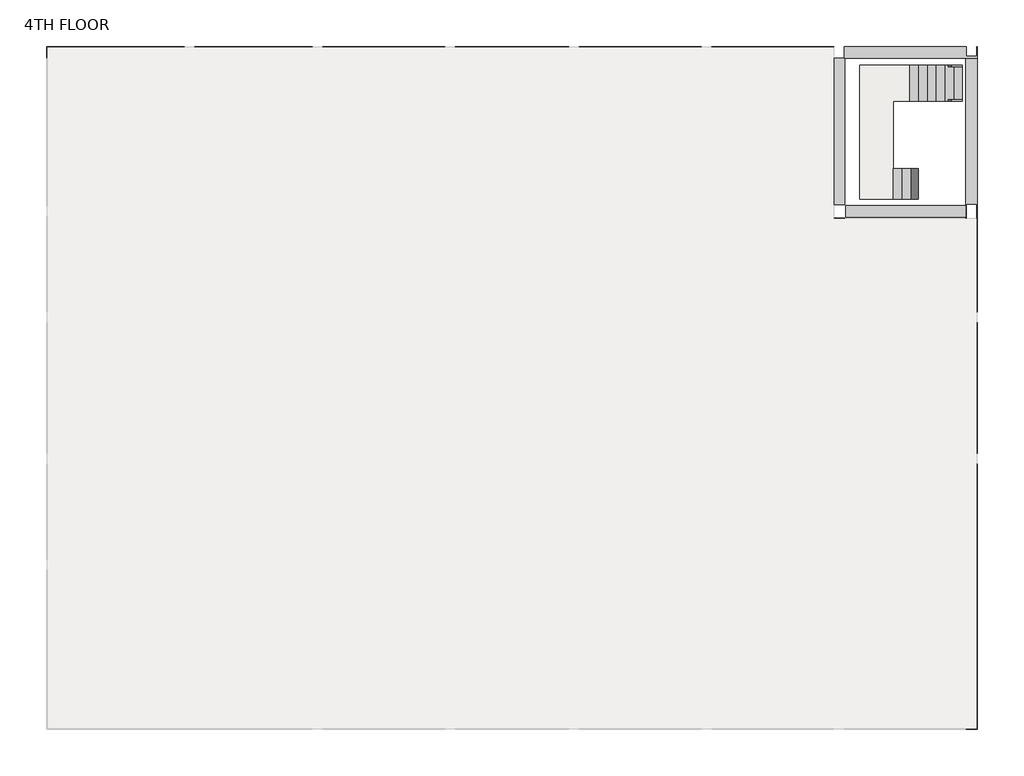
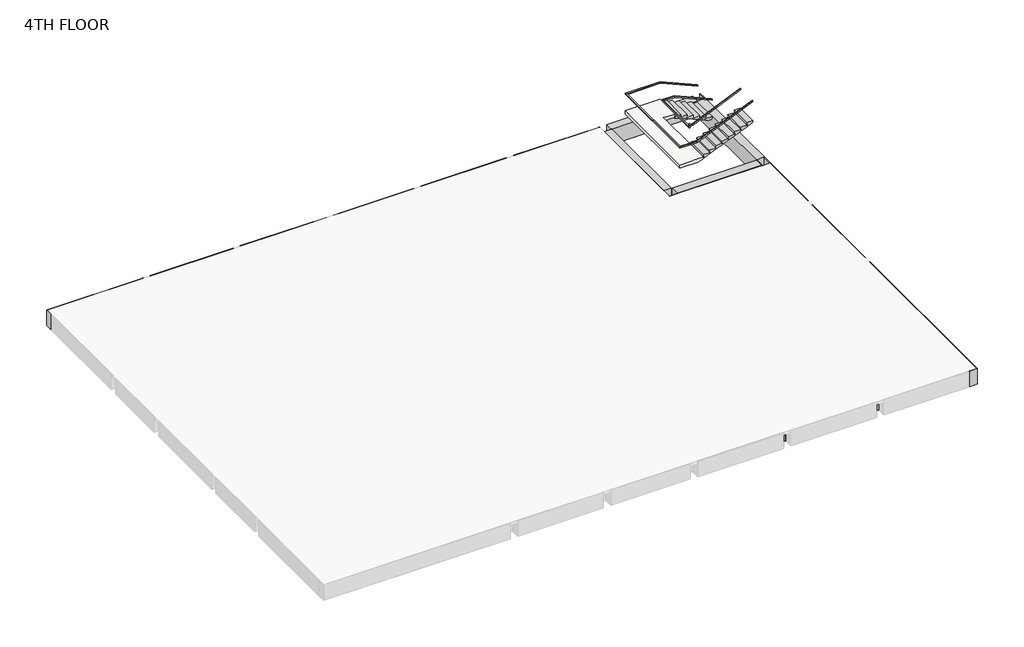
# One storey, part 2 of 2: 5 beams, 2 railings, 2 stair flights, 1 slab.
"""IFC4 building model written with IfcOpenShell, lengths in millimetres."""

from ifc_helpers import new_model, si_unit, frame, origin, place, context, project, spatial, polyline, outline, extrude, faceted_brep, element, save

model = new_model("IFC4")

# Units and contexts
model_context = context("Model", 3, world=origin())
ifc_project = project(units=[si_unit("LENGTHUNIT", "METRE", prefix="MILLI")], contexts=[model_context])

# Site, building, storey
site = spatial("IfcSite", under=ifc_project)
building = spatial("IfcBuilding", under=site)
storey = spatial("IfcBuildingStorey", under=building, Name="4TH FLOOR", Elevation=13716.0)

# Beams
placement = place(None, origin())
element("IfcBeam", 1, ObjectType="M_Concrete-Rectangular Beam : 400 x 800mm", at=placement, inside=storey, context=model_context, shape_type="Brep", body=[
    faceted_brep([(6397.6508981, 16716.9690835, 13716.0), (6397.6508981, 17116.9690835, 13716.0), (6375.4508981, 17116.9690835, 13716.0), (6375.4508981, 16789.9690835, 13716.0), (6019.8508981, 16789.9690835, 13716.0), (6019.8508981, 17116.9690835, 13716.0), (1803.4508981, 17116.9690835, 13716.0), (1803.4508981, 16716.9690835, 13716.0), (1825.6508981, 16716.9690835, 13716.0), (5997.6508981, 16716.9690835, 13716.0), (6397.6508981, 16716.9690835, 12916.0), (1803.4508981, 16716.9690835, 12916.0), (1825.6508981, 16716.9690835, 12916.0), (5997.6508981, 16716.9690835, 12916.0), (6397.6508981, 17116.9690835, 12916.0), (1803.4508981, 17116.9690835, 12916.0), (6019.8508981, 17116.9690835, 12916.0), (6019.8508981, 16789.9690835, 12916.0), (6375.4508981, 16789.9690835, 12916.0), (6375.4508981, 17116.9690835, 12916.0)], [[[0, 1, 2, 3, 4, 5, 6, 7, 8, 9]], [[10, 0, 9, 8, 7, 11, 12, 13]], [[14, 10, 13, 12, 11, 15, 16, 17, 18, 19]], [[1, 14, 19, 2]], [[1, 0, 10, 14]], [[18, 3, 2, 19]], [[3, 18, 17, 4]], [[4, 17, 16, 5]], [[5, 16, 15, 6]], [[7, 6, 15, 11]]]),
    faceted_brep([(-25701.5491019, 16716.9690835, 13716.0), (-25701.5491019, 17116.9690835, 13716.0), (-25701.5491019, 17116.9690835, 12916.0), (-25701.5491019, 16716.9690835, 12916.0), (-25323.7491019, 17094.7690835, 12916.0), (-25323.7491019, 16739.1690835, 12916.0), (-25323.7491019, 16739.1690835, 13563.6), (-25323.7491019, 17094.7690835, 13563.6), (-25679.3491019, 16739.1690835, 12916.0), (-25679.3491019, 16739.1690835, 13563.6), (-25679.3491019, 16716.9690835, 13716.0), (-25679.3491019, 16716.9690835, 13563.6), (-25679.3491019, 17094.7690835, 12916.0), (-25679.3491019, 17094.7690835, 13563.6), (-25679.3491019, 17094.7690835, 13716.0), (-20954.9491019, 16716.9690835, 12916.0), (-20954.9491019, 17116.9690835, 12916.0), (-20954.9491019, 17116.9690835, 13716.0), (-20954.9491019, 17094.7690835, 13716.0), (-20954.9491019, 17094.7690835, 13563.6), (-20954.9491019, 16716.9690835, 13563.6), (-25301.5491019, 16716.9690835, 12916.0), (-20977.1491019, 16716.9690835, 12916.0), (-20977.1491019, 16716.9690835, 13563.6), (-25301.5491019, 16716.9690835, 13563.6)], [[[0, 1, 2, 3]], [[4, 5, 6, 7]], [[5, 8, 9, 6]], [[10, 11, 9, 8, 12, 13, 14]], [[15, 16, 17, 18, 19, 20]], [[1, 0, 10, 14, 18, 17]], [[0, 3, 21, 22, 15, 20, 23, 24, 11, 10]], [[3, 2, 16, 15, 22, 21], [5, 4, 12, 8]], [[2, 1, 17, 16]], [[14, 13, 12, 4, 7, 19, 18]], [[19, 7, 6, 9, 11, 24, 23, 20]]]),
    faceted_brep([(-2768.5491019, 17094.7690835, 13563.6), (1447.8508981, 17094.7690835, 13563.6), (1447.8508981, 17094.7690835, 13716.0), (-2768.5491019, 17094.7690835, 13716.0), (-2768.5491019, 17116.9690835, 12916.0), (-2768.5491019, 16716.9690835, 12916.0), (-2768.5491019, 16716.9690835, 13563.6), (-2768.5491019, 17116.9690835, 13716.0), (1447.8508981, 16716.9690835, 12916.0), (1447.8508981, 17116.9690835, 12916.0), (1447.8508981, 17116.9690835, 13716.0), (1447.8508981, 16716.9690835, 13563.6), (-2746.3491019, 16716.9690835, 12916.0), (1425.6508981, 16716.9690835, 12916.0), (1425.6508981, 16716.9690835, 13563.6), (-2746.3491019, 16716.9690835, 13563.6)], [[[0, 1, 2, 3]], [[4, 5, 6, 0, 3, 7]], [[8, 9, 10, 2, 1, 11]], [[10, 7, 3, 2]], [[5, 12, 13, 8, 11, 14, 15, 6]], [[5, 4, 9, 8, 13, 12]], [[4, 7, 10, 9]], [[1, 0, 6, 15, 14, 11]]]),
    faceted_brep([(-16179.7491019, 17116.9690835, 12916.0), (-16179.7491019, 16716.9690835, 12916.0), (-16179.7491019, 16716.9690835, 13563.6), (-16179.7491019, 17094.7690835, 13563.6), (-16179.7491019, 17094.7690835, 13716.0), (-16179.7491019, 17116.9690835, 13716.0), (-11963.3491019, 16716.9690835, 12916.0), (-11963.3491019, 17116.9690835, 12916.0), (-11963.3491019, 17116.9690835, 13716.0), (-11963.3491019, 17094.7690835, 13716.0), (-11963.3491019, 17094.7690835, 13563.6), (-11963.3491019, 16716.9690835, 13563.6), (-16157.5491019, 16716.9690835, 12916.0), (-11985.5491019, 16716.9690835, 12916.0), (-11985.5491019, 16716.9690835, 13563.6), (-16157.5491019, 16716.9690835, 13563.6)], [[[0, 1, 2, 3, 4, 5]], [[6, 7, 8, 9, 10, 11]], [[8, 5, 4, 9]], [[1, 12, 13, 6, 11, 14, 15, 2]], [[1, 0, 7, 6, 13, 12]], [[0, 5, 8, 7]], [[3, 10, 9, 4]], [[10, 3, 2, 15, 14, 11]]]),
    faceted_brep([(-16535.3491019, 16716.9690835, 12916.0), (-16535.3491019, 17116.9690835, 12916.0), (-16535.3491019, 17116.9690835, 13716.0), (-16535.3491019, 17094.7690835, 13716.0), (-16535.3491019, 17094.7690835, 13563.6), (-16535.3491019, 16716.9690835, 13563.6), (-20599.3491019, 17116.9690835, 13716.0), (-20599.3491019, 17094.7690835, 13716.0), (-20599.3491019, 16716.9690835, 12916.0), (-20577.1491019, 16716.9690835, 12916.0), (-16557.5491019, 16716.9690835, 12916.0), (-16557.5491019, 16716.9690835, 13563.6), (-20577.1491019, 16716.9690835, 13563.6), (-20599.3491019, 16716.9690835, 13563.6), (-20599.3491019, 17116.9690835, 12916.0), (-20599.3491019, 17094.7690835, 13563.6)], [[[0, 1, 2, 3, 4, 5]], [[2, 6, 7, 3]], [[8, 9, 10, 0, 5, 11, 12, 13]], [[1, 0, 10, 9, 8, 14]], [[2, 1, 14, 6]], [[14, 8, 13, 15, 7, 6]], [[15, 4, 3, 7]], [[4, 15, 13, 12, 11, 5]]]),
    faceted_brep([(-11607.7491019, 17116.9690835, 12916.0), (-11607.7491019, 16716.9690835, 12916.0), (-11607.7491019, 16716.9690835, 13563.6), (-11607.7491019, 17094.7690835, 13563.6), (-11607.7491019, 17094.7690835, 13716.0), (-11607.7491019, 17116.9690835, 13716.0), (-7696.1491019, 16716.9690835, 12916.0), (-7696.1491019, 17116.9690835, 12916.0), (-7696.1491019, 17116.9690835, 13716.0), (-7696.1491019, 17094.7690835, 13716.0), (-7696.1491019, 17094.7690835, 13563.6), (-7696.1491019, 16716.9690835, 13563.6), (-11585.5491019, 16716.9690835, 12916.0), (-7718.3491019, 16716.9690835, 12916.0), (-7718.3491019, 16716.9690835, 13563.6), (-11585.5491019, 16716.9690835, 13563.6)], [[[0, 1, 2, 3, 4, 5]], [[6, 7, 8, 9, 10, 11]], [[8, 5, 4, 9]], [[1, 12, 13, 6, 11, 14, 15, 2]], [[1, 0, 7, 6, 13, 12]], [[0, 5, 8, 7]], [[3, 10, 9, 4]], [[10, 3, 2, 15, 14, 11]]]),
    faceted_brep([(-7340.5491019, 17116.9690835, 12916.0), (-7340.5491019, 16716.9690835, 12916.0), (-7340.5491019, 16716.9690835, 13563.6), (-7340.5491019, 17094.7690835, 13563.6), (-7340.5491019, 17094.7690835, 13716.0), (-7340.5491019, 17116.9690835, 13716.0), (-3124.1491019, 16716.9690835, 12916.0), (-3124.1491019, 17116.9690835, 12916.0), (-3124.1491019, 17116.9690835, 13716.0), (-3124.1491019, 17094.7690835, 13716.0), (-3124.1491019, 17094.7690835, 13563.6), (-3124.1491019, 16716.9690835, 13563.6), (-7318.3491019, 16716.9690835, 12916.0), (-3146.3491019, 16716.9690835, 12916.0), (-3146.3491019, 16716.9690835, 13563.6), (-7318.3491019, 16716.9690835, 13563.6)], [[[0, 1, 2, 3, 4, 5]], [[6, 7, 8, 9, 10, 11]], [[8, 5, 4, 9]], [[1, 12, 13, 6, 11, 14, 15, 2]], [[1, 0, 7, 6, 13, 12]], [[0, 5, 8, 7]], [[3, 10, 9, 4]], [[10, 3, 2, 15, 14, 11]]]),
])
element("IfcBeam", 2, ObjectType="M_Concrete-Rectangular Beam : 400 x 800mm", at=placement, inside=storey, context=model_context, shape_type="Brep", body=[
    faceted_brep([(5997.6508981, -6447.8309165, 13716.0), (6397.6508981, -6447.8309165, 13716.0), (6397.6508981, 2718.3690835, 13716.0), (6375.4508981, 2718.3690835, 13716.0), (6375.4508981, -6425.6309165, 13716.0), (5997.6508981, -6425.6309165, 13716.0), (5997.6508981, -6447.8309165, 12916.0), (5997.6508981, -6425.6309165, 13563.6), (5997.6508981, -6047.8309165, 13563.6), (5997.6508981, -961.4309165, 13563.6), (5997.6508981, -561.4309165, 13563.6), (5997.6508981, 2696.1690835, 13563.6), (5997.6508981, 2718.3690835, 13563.6), (5997.6508981, 2718.3690835, 12916.0), (5997.6508981, 2696.1690835, 12916.0), (5997.6508981, -561.4309165, 12916.0), (5997.6508981, -961.4309165, 12916.0), (5997.6508981, -6047.8309165, 12916.0), (6397.6508981, -6447.8309165, 12916.0), (6397.6508981, 2718.3690835, 12916.0), (6375.4508981, -6425.6309165, 12916.0), (6375.4508981, -6070.0309165, 12916.0), (6019.8508981, -6070.0309165, 12916.0), (6019.8508981, -6425.6309165, 12916.0), (6375.4508981, -1015.4309165, 12916.0), (6375.4508981, -507.4309165, 12916.0), (6019.8508981, -507.4309165, 12916.0), (6019.8508981, -1015.4309165, 12916.0), (6375.4508981, 2718.3690835, 13563.6), (6375.4508981, -507.4309165, 13563.6), (6375.4508981, -1015.4309165, 13563.6), (6375.4508981, -6070.0309165, 13563.6), (6375.4508981, -6425.6309165, 13563.6), (6019.8508981, -6425.6309165, 13563.6), (6019.8508981, -6070.0309165, 13563.6), (6019.8508981, -1015.4309165, 13563.6), (6019.8508981, -507.4309165, 13563.6)], [[[0, 1, 2, 3, 4, 5]], [[6, 0, 5, 7, 8, 9, 10, 11, 12, 13, 14, 15, 16, 17]], [[18, 6, 17, 16, 15, 14, 13, 19], [20, 21, 22, 23], [24, 25, 26, 27]], [[1, 18, 19, 2]], [[1, 0, 6, 18]], [[3, 28, 29, 25, 24, 30, 31, 21, 20, 32, 4]], [[4, 32, 20, 23, 33, 7, 5]], [[23, 22, 34, 33]], [[22, 21, 31, 34]], [[19, 13, 12, 28, 3, 2]], [[24, 27, 35, 30]], [[27, 26, 36, 35]], [[26, 25, 29, 36]], [[31, 30, 35, 36, 29, 28, 12, 11, 10, 9, 8, 7, 33, 34]]]),
    faceted_brep([(5997.6508981, 16716.9690835, 12916.0), (5997.6508981, 16716.9690835, 13716.0), (6397.6508981, 16716.9690835, 13716.0), (6397.6508981, 16716.9690835, 12916.0), (5997.6508981, 7950.7690835, 12916.0), (6397.6508981, 7950.7690835, 12916.0), (6397.6508981, 7950.7690835, 13716.0), (6375.4508981, 7950.7690835, 13716.0), (6375.4508981, 7950.7690835, 13563.6), (5997.6508981, 7950.7690835, 13563.6), (5997.6508981, 11630.5690835, 13716.0), (5997.6508981, 11230.5690835, 13716.0), (5997.6508981, 11176.5690835, 13716.0), (6019.8508981, 11176.5690835, 13716.0), (6019.8508981, 11684.5690835, 13716.0), (6375.4508981, 11684.5690835, 13716.0), (6375.4508981, 11176.5690835, 13716.0), (5997.6508981, 11630.5690835, 12916.0), (5997.6508981, 11230.5690835, 12916.0), (5997.6508981, 7972.9690835, 12916.0), (5997.6508981, 7972.9690835, 13563.6), (5997.6508981, 11176.5690835, 13563.6), (6375.4508981, 11176.5690835, 12916.0), (6375.4508981, 11684.5690835, 12916.0), (6019.8508981, 11684.5690835, 12916.0), (6019.8508981, 11176.5690835, 12916.0), (6019.8508981, 11176.5690835, 13563.6), (6375.4508981, 11176.5690835, 13563.6)], [[[0, 1, 2, 3]], [[4, 5, 6, 7, 8, 9]], [[2, 1, 10, 11, 12, 13, 14, 15, 16, 7, 6]], [[1, 0, 17, 18, 19, 4, 9, 20, 21, 12, 11, 10]], [[0, 3, 5, 4, 19, 18, 17], [22, 23, 24, 25]], [[3, 2, 6, 5]], [[22, 25, 26, 27]], [[24, 14, 13, 26, 25]], [[14, 24, 23, 15]], [[8, 27, 26, 21, 20, 9]], [[27, 8, 7, 16, 15, 23, 22]], [[21, 26, 13, 12]]]),
    faceted_brep([(6397.6508981, 7595.1690835, 12916.0), (5997.6508981, 7595.1690835, 12916.0), (5997.6508981, 7595.1690835, 13563.6), (6375.4508981, 7595.1690835, 13563.6), (6375.4508981, 7595.1690835, 13716.0), (6397.6508981, 7595.1690835, 13716.0), (5997.6508981, 3073.9690835, 12916.0), (6397.6508981, 3073.9690835, 12916.0), (6397.6508981, 3073.9690835, 13716.0), (6375.4508981, 3073.9690835, 13716.0), (6375.4508981, 3073.9690835, 13563.6), (5997.6508981, 3073.9690835, 13563.6), (5997.6508981, 7572.9690835, 12916.0), (5997.6508981, 3096.1690835, 12916.0), (5997.6508981, 3096.1690835, 13563.6), (5997.6508981, 7572.9690835, 13563.6)], [[[0, 1, 2, 3, 4, 5]], [[6, 7, 8, 9, 10, 11]], [[8, 5, 4, 9]], [[1, 12, 13, 6, 11, 14, 15, 2]], [[1, 0, 7, 6, 13, 12]], [[0, 5, 8, 7]], [[3, 10, 9, 4]], [[10, 3, 2, 15, 14, 11]]]),
])
element("IfcBeam", 3, ObjectType="M_Concrete-Rectangular Beam : 400 x 800mm", at=placement, inside=storey, context=model_context, shape_type="SweptSolid", body=[
    extrude(outline(polyline([(-2746.3491019, -6047.8309165), (-2768.5491019, -6047.8309165), (-2768.5491019, -6019.2309165), (-3124.1491019, -6019.2309165), (-3124.1491019, -6047.8309165), (-3146.3491019, -6047.8309165), (-3146.3491019, -990.0309165), (-2746.3491019, -990.0309165), (-2746.3491019, -6047.8309165)])), frame((0.0, 0.0, 12916.0), z_axis=(0.0, 0.0, 1.0), x_axis=(1.0, 0.0, 0.0)), (0.0, 0.0, 1.0), 647.6),
    extrude(outline(polyline([(-2768.5491019, 16716.9690835), (-2746.3491019, 16716.9690835), (-2746.3491019, 11659.1690835), (-3146.3491019, 11659.1690835), (-3146.3491019, 16716.9690835), (-3124.1491019, 16716.9690835), (-3124.1491019, 16688.3690835), (-2768.5491019, 16688.3690835), (-2768.5491019, 16716.9690835)])), frame((0.0, 0.0, 12916.0), z_axis=(0.0, 0.0, 1.0), x_axis=(1.0, 0.0, 0.0)), (0.0, 0.0, 1.0), 647.6),
    extrude(outline(polyline([(-3146.3491019, 11201.9690835), (-2746.3491019, 11201.9690835), (-2746.3491019, 8001.5690835), (-3146.3491019, 8001.5690835), (-3146.3491019, 11201.9690835)])), frame((0.0, 0.0, 12916.0), z_axis=(0.0, 0.0, 1.0), x_axis=(1.0, 0.0, 0.0)), (0.0, 0.0, 1.0), 647.6),
    extrude(outline(polyline([(-3146.3491019, 7544.3690835), (-2746.3491019, 7544.3690835), (-2746.3491019, 3124.7690835), (-3146.3491019, 3124.7690835), (-3146.3491019, 7544.3690835)])), frame((0.0, 0.0, 12916.0), z_axis=(0.0, 0.0, 1.0), x_axis=(1.0, 0.0, 0.0)), (0.0, 0.0, 1.0), 647.6),
    extrude(outline(polyline([(-2746.3491019, -532.8309165), (-3146.3491019, -532.8309165), (-3146.3491019, 2667.5690835), (-2746.3491019, 2667.5690835), (-2746.3491019, -532.8309165)])), frame((0.0, 0.0, 12916.0), z_axis=(0.0, 0.0, 1.0), x_axis=(1.0, 0.0, 0.0)), (0.0, 0.0, 1.0), 647.6),
])
element("IfcBeam", 4, ObjectType="M_Concrete-Rectangular Beam : 400 x 800mm", at=placement, inside=storey, context=model_context, shape_type="Brep", body=[
    faceted_brep([(1425.6508981, -990.0309165, 12916.0), (1425.6508981, -6047.8309165, 12916.0), (1425.6508981, -6047.8309165, 13563.6), (1425.6508981, -990.0309165, 13563.6), (1825.6508981, -6047.8309165, 12916.0), (1803.4508981, -6047.8309165, 12916.0), (1803.4508981, -6019.2309165, 12916.0), (1447.8508981, -6019.2309165, 12916.0), (1447.8508981, -6047.8309165, 12916.0), (1825.6508981, -990.0309165, 12916.0), (1825.6508981, -990.0309165, 13563.6), (1825.6508981, -6047.8309165, 13563.6), (1447.8508981, -6047.8309165, 13563.6), (1803.4508981, -6047.8309165, 13563.6), (1803.4508981, -6019.2309165, 13563.6), (1447.8508981, -6019.2309165, 13563.6)], [[[0, 1, 2, 3]], [[4, 5, 6, 7, 8, 1, 0, 9]], [[4, 9, 10, 11]], [[1, 8, 12, 2]], [[6, 5, 13, 14]], [[8, 7, 15, 12]], [[7, 6, 14, 15]], [[5, 4, 11, 13]], [[9, 0, 3, 10]], [[3, 2, 12, 15, 14, 13, 11, 10]]]),
    faceted_brep([(1825.6508981, 16716.9690835, 13716.0), (1825.6508981, 16716.9690835, 12916.0), (1803.4508981, 16716.9690835, 12916.0), (1803.4508981, 16716.9690835, 13716.0), (1803.4508981, 16713.7690835, 12916.0), (1803.4508981, 16713.7690835, 13716.0), (1447.8508981, 16713.7690835, 12916.0), (1447.8508981, 16713.7690835, 13563.6), (1447.8508981, 16713.7690835, 13716.0), (1447.8508981, 16716.9690835, 12916.0), (1447.8508981, 16716.9690835, 13563.6), (1425.6508981, 16716.9690835, 12916.0), (1425.6508981, 16716.9690835, 13563.6), (1425.6508981, 11659.1690835, 12916.0), (1825.6508981, 11659.1690835, 12916.0), (1825.6508981, 11659.1690835, 13716.0), (1447.8508981, 11659.1690835, 13716.0), (1447.8508981, 11659.1690835, 13563.6), (1425.6508981, 11659.1690835, 13563.6)], [[[0, 1, 2, 3]], [[4, 5, 3, 2]], [[5, 4, 6, 7, 8]], [[6, 9, 10, 7]], [[9, 11, 12, 10]], [[13, 14, 15, 16, 17, 18]], [[0, 3, 5, 8, 16, 15]], [[11, 13, 18, 12]], [[2, 1, 14, 13, 11, 9, 6, 4]], [[1, 0, 15, 14]], [[17, 7, 10, 12, 18]], [[7, 17, 16, 8]]]),
    faceted_brep([(1825.6508981, 11201.9690835, 12916.0), (1425.6508981, 11201.9690835, 12916.0), (1425.6508981, 11201.9690835, 13563.6), (1447.8508981, 11201.9690835, 13563.6), (1447.8508981, 11201.9690835, 13716.0), (1825.6508981, 11201.9690835, 13716.0), (1425.6508981, 8001.5690835, 12916.0), (1825.6508981, 8001.5690835, 12916.0), (1825.6508981, 8001.5690835, 13563.6), (1425.6508981, 8001.5690835, 13563.6), (1447.8508981, 11176.5690835, 13716.0), (1825.6508981, 11176.5690835, 13716.0), (1825.6508981, 11176.5690835, 13563.6), (1447.8508981, 11176.5690835, 13563.6)], [[[0, 1, 2, 3, 4, 5]], [[6, 7, 8, 9]], [[5, 4, 10, 11]], [[1, 6, 9, 2]], [[1, 0, 7, 6]], [[0, 5, 11, 12, 8, 7]], [[12, 13, 3, 2, 9, 8]], [[13, 10, 4, 3]], [[10, 13, 12, 11]]]),
    faceted_brep([(1825.6508981, 7544.3690835, 12916.0), (1425.6508981, 7544.3690835, 12916.0), (1425.6508981, 7544.3690835, 13563.6), (1825.6508981, 7544.3690835, 13563.6), (1425.6508981, 3124.7690835, 12916.0), (1825.6508981, 3124.7690835, 12916.0), (1825.6508981, 3124.7690835, 13563.6), (1425.6508981, 3124.7690835, 13563.6)], [[[0, 1, 2, 3]], [[4, 5, 6, 7]], [[1, 4, 7, 2]], [[1, 0, 5, 4]], [[5, 0, 3, 6]], [[3, 2, 7, 6]]]),
    faceted_brep([(1425.6508981, -532.8309165, 12916.0), (1825.6508981, -532.8309165, 12916.0), (1825.6508981, -532.8309165, 13563.6), (1425.6508981, -532.8309165, 13563.6), (1425.6508981, 2667.5690835, 12916.0), (1425.6508981, 2667.5690835, 13563.6), (1825.6508981, 2667.5690835, 12916.0), (1825.6508981, 2667.5690835, 13563.6)], [[[0, 1, 2, 3]], [[4, 0, 3, 5]], [[1, 0, 4, 6]], [[1, 6, 7, 2]], [[6, 4, 5, 7]], [[3, 2, 7, 5]]]),
])
element("IfcBeam", 5, ObjectType="M_Concrete-Rectangular Beam : 400 x 800mm", at=placement, inside=storey, context=model_context, shape_type="SweptSolid", body=[
    extrude(outline(polyline([(-25301.5491019, 11608.3690835), (-25301.5491019, 11630.5690835), (-21005.7491019, 11630.5690835), (-21005.7491019, 11230.5690835), (-25301.5491019, 11230.5690835), (-25301.5491019, 11252.7690835), (-25247.5491019, 11252.7690835), (-25247.5491019, 11608.3690835), (-25301.5491019, 11608.3690835)])), frame((0.0, 0.0, 12916.0), z_axis=(0.0, 0.0, 1.0), x_axis=(1.0, 0.0, 0.0)), (0.0, 0.0, 1.0), 647.6),
    extrude(outline(polyline([(5997.6508981, 11630.5690835), (5997.6508981, 11230.5690835), (1854.2508981, 11230.5690835), (1854.2508981, 11630.5690835), (5997.6508981, 11630.5690835)])), frame((0.0, 0.0, 12916.0), z_axis=(0.0, 0.0, 1.0), x_axis=(1.0, 0.0, 0.0)), (0.0, 0.0, 1.0), 800.0),
    extrude(outline(polyline([(-20548.5491019, 11230.5690835), (-20548.5491019, 11630.5690835), (-16586.1491019, 11630.5690835), (-16586.1491019, 11230.5690835), (-20548.5491019, 11230.5690835)])), frame((0.0, 0.0, 12916.0), z_axis=(0.0, 0.0, 1.0), x_axis=(1.0, 0.0, 0.0)), (0.0, 0.0, 1.0), 647.6),
    extrude(outline(polyline([(-16128.9491019, 11230.5690835), (-16128.9491019, 11630.5690835), (-12014.1491019, 11630.5690835), (-12014.1491019, 11230.5690835), (-16128.9491019, 11230.5690835)])), frame((0.0, 0.0, 12916.0), z_axis=(0.0, 0.0, 1.0), x_axis=(1.0, 0.0, 0.0)), (0.0, 0.0, 1.0), 647.6),
    extrude(outline(polyline([(-11556.9491019, 11230.5690835), (-11556.9491019, 11630.5690835), (-7746.9491019, 11630.5690835), (-7746.9491019, 11230.5690835), (-11556.9491019, 11230.5690835)])), frame((0.0, 0.0, 12916.0), z_axis=(0.0, 0.0, 1.0), x_axis=(1.0, 0.0, 0.0)), (0.0, 0.0, 1.0), 647.6),
    extrude(outline(polyline([(-7289.7491019, 11230.5690835), (-7289.7491019, 11630.5690835), (-3174.9491019, 11630.5690835), (-3174.9491019, 11230.5690835), (-7289.7491019, 11230.5690835)])), frame((0.0, 0.0, 12916.0), z_axis=(0.0, 0.0, 1.0), x_axis=(1.0, 0.0, 0.0)), (0.0, 0.0, 1.0), 647.6),
    extrude(outline(polyline([(-2717.7491019, 11230.5690835), (-2717.7491019, 11630.5690835), (1397.0508981, 11630.5690835), (1397.0508981, 11230.5690835), (-2717.7491019, 11230.5690835)])), frame((0.0, 0.0, 12916.0), z_axis=(0.0, 0.0, 1.0), x_axis=(1.0, 0.0, 0.0)), (0.0, 0.0, 1.0), 647.6),
])

# Railings
element("IfcRailing", 6, ObjectType="Handrail", at=placement, inside=storey, context=model_context, shape_type="Brep", body=[
    faceted_brep([(5878.2258195, 16426.305974, 14760.575), (5878.2258195, 16426.305974, 14705.3359813), (5878.2258195, 16477.105974, 14705.3359813), (5878.2258195, 16477.105974, 14760.575), (4049.4258195, 16426.305974, 15541.625), (4039.0320197, 16426.305974, 15490.825), (4039.0320197, 16477.105974, 15490.825), (4049.4258195, 16477.105974, 15541.625), (2398.4258195, 16426.305974, 15541.625), (2398.4258195, 16426.305974, 15490.825), (2347.6258195, 16477.105974, 15490.825), (2347.6258195, 16477.105974, 15541.625), (2398.4258195, 11896.1816424, 15541.625), (2398.4258195, 11896.1816424, 15490.825), (2347.6258195, 11845.3816424, 15490.825), (2347.6258195, 11845.3816424, 15541.625), (3188.2923097, 11896.1816424, 15541.625), (3198.6861096, 11896.1816424, 15490.825), (3198.6861096, 11845.3816424, 15490.825), (3188.2923097, 11845.3816424, 15541.625), (5931.4923097, 11896.1816424, 16713.2), (5931.4923097, 11845.3816424, 16713.2), (5931.4923097, 11845.3816424, 16657.9609813), (5931.4923097, 11896.1816424, 16657.9609813)], [[[0, 1, 2, 3]], [[1, 0, 4, 5]], [[2, 1, 5, 6]], [[3, 2, 6, 7]], [[0, 3, 7, 4]], [[5, 4, 8, 9]], [[6, 5, 9, 10]], [[7, 6, 10, 11]], [[4, 7, 11, 8]], [[9, 8, 12, 13]], [[10, 9, 13, 14]], [[11, 10, 14, 15]], [[8, 11, 15, 12]], [[13, 12, 16, 17]], [[14, 13, 17, 18]], [[15, 14, 18, 19]], [[12, 15, 19, 16]], [[20, 21, 22, 23]], [[17, 16, 20, 23]], [[18, 17, 23, 22]], [[19, 18, 22, 21]], [[16, 19, 21, 20]]]),
])
element("IfcRailing", 7, ObjectType="Handrail", at=placement, inside=storey, context=model_context, shape_type="Brep", body=[
    faceted_brep([(5878.2258195, 15223.6852874, 14760.575), (5878.2258195, 15223.6852874, 14705.3359813), (5878.2258195, 15274.4852874, 14705.3359813), (5878.2258195, 15274.4852874, 14760.575), (4049.4258195, 15223.6852874, 15541.625), (4039.0320197, 15223.6852874, 15490.825), (4039.0320197, 15274.4852874, 15490.825), (4049.4258195, 15274.4852874, 15541.625), (3493.0923097, 15223.6852874, 15541.625), (3493.0923097, 15223.6852874, 15490.825), (3442.2923097, 15274.4852874, 15490.825), (3442.2923097, 15274.4852874, 15541.625), (3493.0923097, 12985.9409784, 15541.625), (3493.0923097, 12935.1409784, 15490.825), (3442.2923097, 12935.1409784, 15490.825), (3442.2923097, 12985.9409784, 15541.625), (3493.0923097, 12985.9409784, 15704.34375), (3493.0923097, 12935.1409784, 15653.54375), (3442.2923097, 12935.1409784, 15653.54375), (3442.2923097, 12985.9409784, 15704.34375), (3493.0923097, 12909.7409784, 15704.34375), (3493.0923097, 12909.7409784, 15653.54375), (3442.2923097, 12858.9409784, 15653.54375), (3442.2923097, 12858.9409784, 15704.34375), (3569.2923097, 12909.7409784, 15704.34375), (3579.6861096, 12909.7409784, 15653.54375), (3579.6861096, 12858.9409784, 15653.54375), (3569.2923097, 12858.9409784, 15704.34375), (5931.4923097, 12909.7409784, 16713.2), (5931.4923097, 12858.9409784, 16713.2), (5931.4923097, 12858.9409784, 16657.9609813), (5931.4923097, 12909.7409784, 16657.9609813)], [[[0, 1, 2, 3]], [[1, 0, 4, 5]], [[2, 1, 5, 6]], [[3, 2, 6, 7]], [[0, 3, 7, 4]], [[5, 4, 8, 9]], [[6, 5, 9, 10]], [[7, 6, 10, 11]], [[4, 7, 11, 8]], [[9, 8, 12, 13]], [[10, 9, 13, 14]], [[11, 10, 14, 15]], [[8, 11, 15, 12]], [[13, 12, 16, 17]], [[14, 13, 17, 18]], [[15, 14, 18, 19]], [[12, 15, 19, 16]], [[17, 16, 20, 21]], [[18, 17, 21, 22]], [[19, 18, 22, 23]], [[16, 19, 23, 20]], [[21, 20, 24, 25]], [[22, 21, 25, 26]], [[23, 22, 26, 27]], [[20, 23, 27, 24]], [[28, 29, 30, 31]], [[25, 24, 28, 31]], [[26, 25, 31, 30]], [[27, 26, 30, 29]], [[24, 27, 29, 28]]]),
])

# Slab
element("IfcSlab", 8, ObjectType="7\" Thickness", at=placement, inside=storey, context=model_context, shape_type="Brep", body=[
    faceted_brep([(4049.4258195, 16477.105974, 14627.225), (4049.4258195, 15223.6852874, 14627.225), (4030.3758195, 15223.6852874, 14497.05), (4030.3758195, 16477.105974, 14497.05), (2347.6258195, 16477.105974, 14627.225), (2347.6258195, 11845.3816424, 14627.225), (3257.5052912, 11845.3816424, 14627.225), (3493.0923097, 11845.3816424, 14627.225), (3512.1423097, 11845.3816424, 14627.225), (3512.1423097, 12909.7409784, 14627.225), (3493.0923097, 12909.7409784, 14627.225), (3493.0923097, 15223.6852874, 14627.225), (3980.212838, 15223.6852874, 14627.225), (3980.212838, 16477.105974, 14627.225), (4030.3758195, 15223.6852874, 14428.0012267), (4030.3758195, 16477.105974, 14428.0012267), (3980.212838, 16477.105974, 14449.425), (2347.6258195, 16477.105974, 14449.425), (2347.6258195, 11845.3816424, 14449.425), (3257.5052912, 11845.3816424, 14449.425), (3493.0923097, 11845.3816424, 14550.0402892), (3512.1423097, 11845.3816424, 14558.1762267), (3512.1423097, 12909.7409784, 14558.1762267), (3493.0923097, 12909.7409784, 14550.0402892), (3493.0923097, 12909.7409784, 14449.425), (3493.0923097, 15223.6852874, 14449.425), (3980.212838, 15223.6852874, 14449.425), (3257.5052912, 12909.7409784, 14449.425)], [[[0, 1, 2, 3]], [[4, 5, 6, 7, 8, 9, 10, 11, 12, 1, 0, 13]], [[3, 2, 14, 15]], [[0, 3, 15, 16, 17, 4, 13]], [[5, 4, 17, 18]], [[5, 18, 19, 20, 7, 6]], [[8, 7, 20, 21]], [[9, 8, 21, 22]], [[10, 9, 22, 23]], [[11, 10, 23, 24, 25]], [[2, 1, 12, 11, 25, 26, 14]], [[24, 27, 19, 18, 17, 16, 26, 25]], [[27, 24, 23]], [[26, 16, 15, 14]], [[19, 27, 23, 22, 21, 20]]]),
])

# Stair flights
element("IfcStairFlight", 9, ObjectType="3/4\" Nosing", at=placement, inside=storey, context=model_context, shape_type="Brep", body=[
    faceted_brep([(5878.2258195, 16477.105974, 13846.175), (5878.2258195, 15223.6852874, 13846.175), (5859.1758195, 15223.6852874, 13716.0), (5859.1758195, 16477.105974, 13716.0), (5554.3758195, 16477.105974, 13846.175), (5554.3758195, 15223.6852874, 13846.175), (5554.3758195, 15223.6852874, 13777.1262267), (5697.5006429, 15223.6852874, 13716.0), (5697.5006429, 16477.105974, 13716.0), (5554.3758195, 16477.105974, 13777.1262267), (5573.4258195, 15223.6852874, 13976.35), (5573.4258195, 16477.105974, 13976.35), (5249.5758195, 16477.105974, 13976.35), (5249.5758195, 15223.6852874, 13976.35), (5249.5758195, 15223.6852874, 13907.3012267), (5249.5758195, 16477.105974, 13907.3012267), (5268.6258195, 15223.6852874, 14106.525), (5268.6258195, 16477.105974, 14106.525), (4944.7758195, 16477.105974, 14106.525), (4944.7758195, 15223.6852874, 14106.525), (4944.7758195, 15223.6852874, 14037.4762267), (4944.7758195, 16477.105974, 14037.4762267), (4963.8258195, 15223.6852874, 14236.7), (4963.8258195, 16477.105974, 14236.7), (4639.9758195, 16477.105974, 14236.7), (4639.9758195, 15223.6852874, 14236.7), (4639.9758195, 15223.6852874, 14167.6512267), (4639.9758195, 16477.105974, 14167.6512267), (4659.0258195, 15223.6852874, 14366.875), (4659.0258195, 16477.105974, 14366.875), (4335.1758195, 16477.105974, 14366.875), (4335.1758195, 15223.6852874, 14366.875), (4335.1758195, 15223.6852874, 14297.8262267), (4335.1758195, 16477.105974, 14297.8262267), (4030.3758195, 15223.6852874, 14497.05), (4049.4258195, 15223.6852874, 14497.05), (4354.2258195, 15223.6852874, 14497.05), (4354.2258195, 16477.105974, 14497.05), (4049.4258195, 16477.105974, 14497.05), (4030.3758195, 16477.105974, 14497.05), (4030.3758195, 15223.6852874, 14428.0012267), (4049.4258195, 15223.6852874, 14419.8652892), (4049.4258195, 16477.105974, 14419.8652892), (4030.3758195, 16477.105974, 14428.0012267)], [[[0, 1, 2, 3]], [[1, 0, 4, 5]], [[1, 5, 6, 7, 2]], [[4, 0, 3, 8, 9]], [[10, 11, 12, 13]], [[10, 13, 14, 6, 5]], [[12, 11, 4, 9, 15]], [[5, 4, 11, 10]], [[16, 17, 18, 19]], [[16, 19, 20, 14, 13]], [[18, 17, 12, 15, 21]], [[13, 12, 17, 16]], [[22, 23, 24, 25]], [[22, 25, 26, 20, 19]], [[24, 23, 18, 21, 27]], [[19, 18, 23, 22]], [[28, 29, 30, 31]], [[28, 31, 32, 26, 25]], [[30, 29, 24, 27, 33]], [[25, 24, 29, 28]], [[34, 35, 36, 37, 38, 39]], [[35, 34, 40, 41]], [[38, 37, 30, 33, 42]], [[34, 39, 43, 40]], [[31, 30, 37, 36]], [[3, 2, 7, 8]], [[8, 7, 6, 14, 20, 26, 32, 41, 40, 43, 42, 33, 27, 21, 15, 9]], [[36, 35, 41, 32, 31]], [[39, 38, 42, 43]]]),
])
element("IfcStairFlight", 10, ObjectType="3/4\" Nosing", at=placement, inside=storey, context=model_context, shape_type="Brep", body=[
    faceted_brep([(3493.0923097, 11845.3816424, 14757.4), (3493.0923097, 12909.7409784, 14757.4), (3512.1423097, 12909.7409784, 14627.225), (3512.1423097, 11845.3816424, 14627.225), (3816.9423097, 11845.3816424, 14757.4), (3816.9423097, 12909.7409784, 14757.4), (3816.9423097, 12909.7409784, 14688.3512267), (3512.1423097, 12909.7409784, 14558.1762267), (3512.1423097, 11845.3816424, 14558.1762267), (3816.9423097, 11845.3816424, 14688.3512267), (3797.8923097, 12909.7409784, 14887.575), (3797.8923097, 11845.3816424, 14887.575), (4121.7423097, 11845.3816424, 14887.575), (4121.7423097, 12909.7409784, 14887.575), (4121.7423097, 12909.7409784, 14818.5262267), (4121.7423097, 11845.3816424, 14818.5262267), (4102.6923097, 12909.7409784, 15017.75), (4102.6923097, 11845.3816424, 15017.75), (4426.5423097, 11845.3816424, 15017.75), (4426.5423097, 12909.7409784, 15017.75), (4426.5423097, 12909.7409784, 14948.7012267), (4426.5423097, 11845.3816424, 14948.7012267), (4407.4923097, 12909.7409784, 15147.925), (4407.4923097, 11845.3816424, 15147.925), (4731.3423097, 11845.3816424, 15147.925), (4731.3423097, 12909.7409784, 15147.925), (4731.3423097, 12909.7409784, 15078.8762267), (4731.3423097, 11845.3816424, 15078.8762267), (4712.2923097, 12909.7409784, 15278.1), (4712.2923097, 11845.3816424, 15278.1), (5036.1423097, 11845.3816424, 15278.1), (5036.1423097, 12909.7409784, 15278.1), (5036.1423097, 12909.7409784, 15209.0512267), (5036.1423097, 11845.3816424, 15209.0512267), (5017.0923097, 12909.7409784, 15408.275), (5017.0923097, 11845.3816424, 15408.275), (5340.9423097, 11845.3816424, 15408.275), (5340.9423097, 12909.7409784, 15408.275), (5340.9423097, 12909.7409784, 15339.2262267), (5340.9423097, 11845.3816424, 15339.2262267), (5321.8923097, 12909.7409784, 15538.45), (5321.8923097, 11845.3816424, 15538.45), (5645.7423097, 11845.3816424, 15538.45), (5645.7423097, 12909.7409784, 15538.45), (5645.7423097, 12909.7409784, 15469.4012267), (5645.7423097, 11845.3816424, 15469.4012267), (5626.6923097, 12909.7409784, 15668.625), (5626.6923097, 11845.3816424, 15668.625), (5931.4923097, 11845.3816424, 15668.625), (5931.4923097, 12909.7409784, 15668.625), (5931.4923097, 12909.7409784, 15591.4402892), (5931.4923097, 11845.3816424, 15591.4402892)], [[[0, 1, 2, 3]], [[1, 0, 4, 5]], [[1, 5, 6, 7, 2]], [[3, 2, 7, 8]], [[4, 0, 3, 8, 9]], [[10, 11, 12, 13]], [[10, 13, 14, 6, 5]], [[12, 11, 4, 9, 15]], [[11, 10, 5, 4]], [[16, 17, 18, 19]], [[16, 19, 20, 14, 13]], [[18, 17, 12, 15, 21]], [[17, 16, 13, 12]], [[22, 23, 24, 25]], [[22, 25, 26, 20, 19]], [[24, 23, 18, 21, 27]], [[23, 22, 19, 18]], [[28, 29, 30, 31]], [[28, 31, 32, 26, 25]], [[30, 29, 24, 27, 33]], [[29, 28, 25, 24]], [[34, 35, 36, 37]], [[34, 37, 38, 32, 31]], [[36, 35, 30, 33, 39]], [[35, 34, 31, 30]], [[40, 41, 42, 43]], [[40, 43, 44, 38, 37]], [[42, 41, 36, 39, 45]], [[41, 40, 37, 36]], [[46, 47, 48, 49]], [[46, 49, 50, 44, 43]], [[48, 47, 42, 45, 51]], [[49, 48, 51, 50]], [[47, 46, 43, 42]], [[7, 6, 14, 20, 26, 32, 38, 44, 50, 51, 45, 39, 33, 27, 21, 15, 9, 8]]]),
])

save(model, "model.ifc")

# Revit data of these elements
# Type "M_Concrete-Rectangular Beam : 400 x 800mm"
#   Length [instance default] = 5' - 0"
#   b = 1' - 3.74803"
#   h = 2' - 7.49606"
#   Structural Material [instance default] = Concrete, Cast-in-Place gray
#   Assembly Code = ""
# Type "Handrail"
#   Assembly Code = "C2010400"
#   built-in parameter 1008612 = 0.0416667 (stored number, unit not read)
#   built-in parameter 1008611 = 0.0416667 (stored number, unit not read)
#   built-in parameter 1008609 = 0.333333 (stored number, unit not read)
#   built-in parameter 1008604 = 0.166667 (stored number, unit not read)
#   built-in parameter 1008603 = 0.166667 (stored number, unit not read)
#   Railing Height = 3' - 0"
#   built-in parameter 1008630 = 2
#   built-in parameter 1008610 = 2
#   built-in parameter 1008618 = Baluster - Square : 3/4"
# Elements 1, 2 (IfcBeam, "M_Concrete-Rectangular Beam : 400 x 800mm")
#   Structural Material = Concrete, Cast-in-Place gray
#   Phase Created = New Construction
#   Materials on its faces: "Concrete, Cast-in-Place gray"
# Elements 3, 4, 5 (IfcBeam, "M_Concrete-Rectangular Beam : 400 x 800mm")
#   Comments = ""
#   Structural Material = Concrete, Cast-in-Place gray
#   Phase Created = New Construction
#   Materials on its faces: "Concrete, Cast-in-Place gray"
# Elements 6, 7 (IfcRailing, "Handrail")
#   Phase Created = New Construction
# Element 8 (IfcSlab, "7\" Thickness")
#   Phase Created = New Construction
#   Materials on its faces: "Concrete, Cast-in-Place gray"
# Elements 9, 10 (IfcStairFlight, "3/4\" Nosing")
#   Phase Created = New Construction
#   Materials on its faces: "Concrete, Cast-in-Place gray"
# Materials
#   "Concrete, Cast-in-Place gray": class "Concrete", colour RGB 192 192 192, transparency 0, Description = "Cast-in-place concrete", Cost = 0
